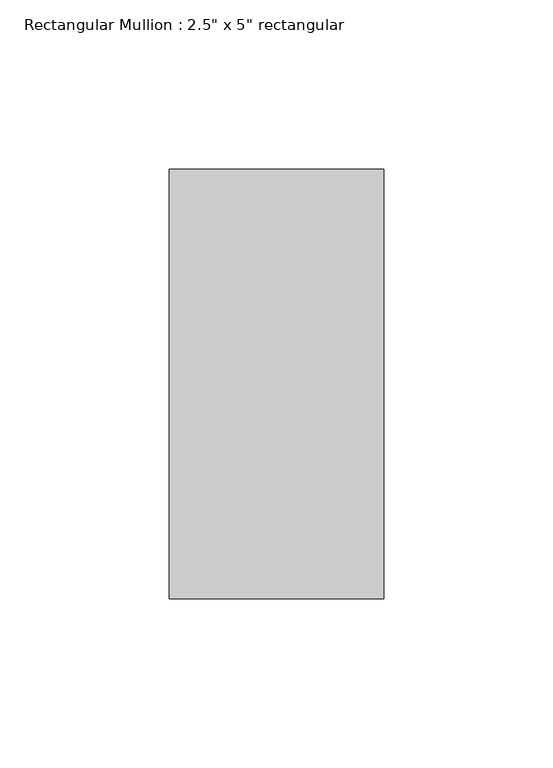
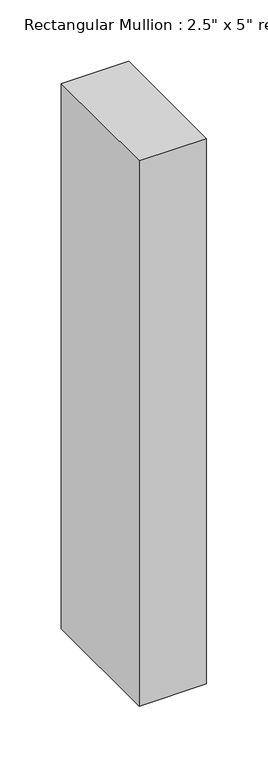
"""IFC4 building model written with IfcOpenShell, lengths in millimetres: member geometry."""

from ifc_helpers import new_model, si_unit, frame, origin, place, context, project, spatial, polyline, outline, extrude, source, transform, mapped, element, save


def member_94e27682(model_context):
    return source(origin(), model_context, "Body", "SweptSolid", [
        extrude(outline(polyline([(0.0, 63.5), (0.0, -63.5), (-63.5, -63.5), (-63.5, 63.5), (0.0, 63.5)])), frame((0.0, 0.0, -544.1386718), z_axis=(0.0, 0.0, 1.0), x_axis=(1.0, 0.0, 0.0)), (0.0, 0.0, 1.0), 544.1386718),
    ])


if __name__ == "__main__":
    model = new_model("IFC4")
    model_context = context("Model", 3, world=origin())
    ifc_project = project(units=[si_unit("LENGTHUNIT", "METRE", prefix="MILLI")], contexts=[model_context])
    site = spatial("IfcSite", under=ifc_project)
    building = spatial("IfcBuilding", under=site)
    placement = place(None, origin())
    member_shape = member_94e27682(model_context)
    element("IfcMember", 1, ObjectType="Rectangular Mullion : 2.5\" x 5\" rectangular", at=placement, inside=building, context=model_context, shape_type="MappedRepresentation", body=[
        mapped(member_shape, transform((0.0, 0.0, 0.0), x_axis=(1.0, 0.0, 0.0), y_axis=(0.0, 1.0, 0.0), z_axis=(0.0, 0.0, 1.0))),
    ])
    save(model, "model.ifc")

# Revit data of these elements
# Type "Rectangular Mullion : 2.5\" x 5\" rectangular"
#   built-in parameter 1007304 = 0.416667 (stored number, unit not read)
#   built-in parameter 1007301 = 0.104167 (stored number, unit not read)
#   built-in parameter 1007300 = 0.104167 (stored number, unit not read)
# Element 1 (IfcMember, "Rectangular Mullion : 2.5\" x 5\" rectangular")
#   Materials on its faces: "Aluminum"
# Materials
#   "Aluminum": class "Metal", colour RGB 247 247 247, transparency 0, Description = "Aluminum 6061", Cost = 0
